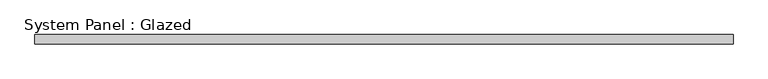
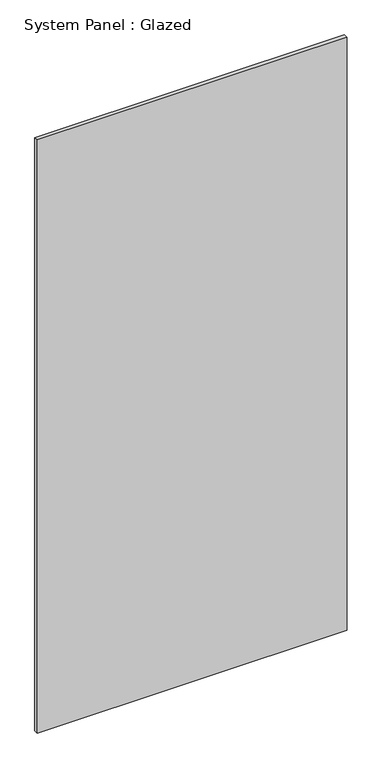
"""IFC4 building model written with IfcOpenShell, lengths in millimetres: plate geometry, System Panel : Glazed."""

from ifc_helpers import new_model, si_unit, origin, origin_with_axes, place, context, project, spatial, polyline, outline, extrude, source, transform, mapped, element, save


def system_panel_glazed_b7adf6b9(model_context):
    return source(origin(), model_context, "Body", "SweptSolid", [
        extrude(outline(polyline([(948.2879709, 19.05), (-948.2879709, 19.05), (-948.2879709, 44.45), (948.2879709, 44.45), (948.2879709, 19.05)])), origin_with_axes(), (0.0, 0.0, 1.0), 3835.4),
    ])


if __name__ == "__main__":
    model = new_model("IFC4")
    model_context = context("Model", 3, world=origin())
    ifc_project = project(units=[si_unit("LENGTHUNIT", "METRE", prefix="MILLI")], contexts=[model_context])
    site = spatial("IfcSite", under=ifc_project)
    building = spatial("IfcBuilding", under=site)
    placement = place(None, origin())
    system_panel_glazed_shape = system_panel_glazed_b7adf6b9(model_context)
    element("IfcPlate", 1, ObjectType="System Panel : Glazed", at=placement, inside=building, context=model_context, shape_type="MappedRepresentation", body=[
        mapped(system_panel_glazed_shape, transform((0.0, 0.0, 0.0), x_axis=(1.0, 0.0, 0.0), y_axis=(0.0, 1.0, 0.0), z_axis=(0.0, 0.0, 1.0))),
    ])
    save(model, "model.ifc")

# Revit data of these elements
# Type "System Panel : Glazed"
#   Construction Type Id = "GSP4R"
#   Analytic Construction = "1/8 in Pilkington single glazing"
#   Visual Light Transmittance = 0.9
#   Solar Heat Gain Coefficient = 0.86
#   Heat Transfer Coefficient (U) = 1.18115 BTU/(h·ft²·°F)
# Element 1 (IfcPlate, "System Panel : Glazed")
#   Materials on its faces: "Glass"
# Materials
#   "Glass": class "Glass", colour RGB 0 128 192, transparency 0.75, Description = "Soda Lime Glass", Cost = 0
